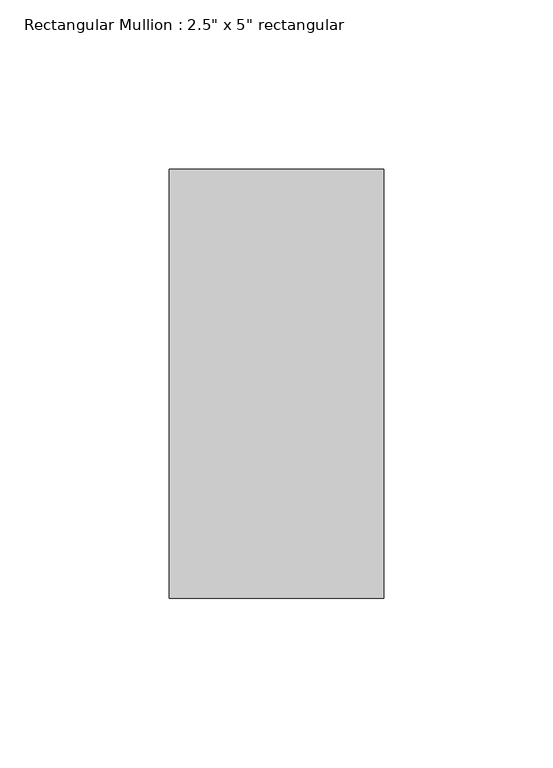
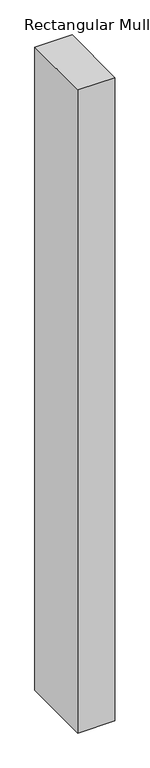
"""IFC4 building model written with IfcOpenShell, lengths in millimetres: member geometry."""

from ifc_helpers import new_model, si_unit, frame, origin, place, context, project, spatial, polyline, outline, extrude, source, transform, mapped, element, save


def member_9e1336f4(model_context):
    return source(origin(), model_context, "Body", "SweptSolid", [
        extrude(outline(polyline([(0.0, 63.5), (0.0, -63.5), (-63.5, -63.5), (-63.5, 63.5), (0.0, 63.5)])), frame((0.0, 0.0, -1162.0499998), z_axis=(0.0, 0.0, 1.0), x_axis=(1.0, 0.0, 0.0)), (0.0, 0.0, 1.0), 1162.0499998),
    ])


if __name__ == "__main__":
    model = new_model("IFC4")
    model_context = context("Model", 3, world=origin())
    ifc_project = project(units=[si_unit("LENGTHUNIT", "METRE", prefix="MILLI")], contexts=[model_context])
    site = spatial("IfcSite", under=ifc_project)
    building = spatial("IfcBuilding", under=site)
    placement = place(None, origin())
    member_shape = member_9e1336f4(model_context)
    element("IfcMember", 1, ObjectType="Rectangular Mullion : 2.5\" x 5\" rectangular", at=placement, inside=building, context=model_context, shape_type="MappedRepresentation", body=[
        mapped(member_shape, transform((0.0, 0.0, 0.0), x_axis=(1.0, 0.0, 0.0), y_axis=(0.0, 1.0, 0.0), z_axis=(0.0, 0.0, 1.0))),
    ])
    save(model, "model.ifc")

# Revit data of these elements
# Type "Rectangular Mullion : 2.5\" x 5\" rectangular"
#   built-in parameter 1007304 = 0.416667 (stored number, unit not read)
#   built-in parameter 1007301 = 0.104167 (stored number, unit not read)
#   built-in parameter 1007300 = 0.104167 (stored number, unit not read)
# Element 1 (IfcMember, "Rectangular Mullion : 2.5\" x 5\" rectangular")
#   Materials on its faces: "BLACK COLOUR"
# Materials
#   "BLACK COLOUR": class "Generic", colour RGB 120 120 120, transparency 0, Cost = 0
